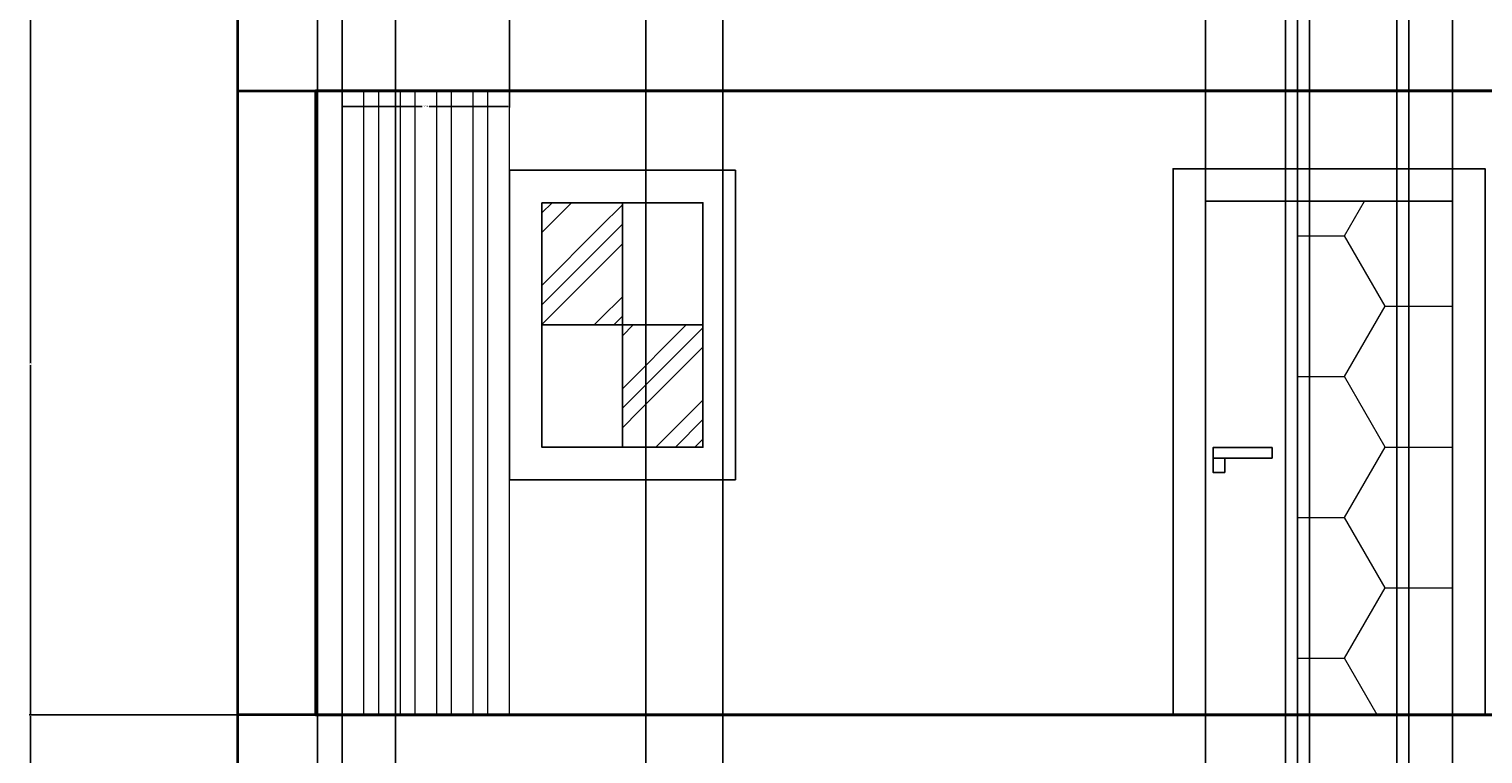
# Model space of a CAD drawing. Units: inches. Extents: x -8 to 554, y -200 to 499.
# Tile 6 of 12: x -8 to 216, y 121 to 233. Entities that reach past the tile are written whole.
import ezdxf

# ---------------------------------------------------------------- set-up
doc = ezdxf.new("R2010")
doc.units = ezdxf.units.IN
doc.header["$MEASUREMENT"] = 0
for name, color, linetype, lineweight in [('A-ANNO-DIMS', 2, 'Continuous', 18), ('A-DOOR', 3, 'Continuous', 25), ('A-DOOR-PATT', 252, 'Continuous', 13), ('A-FLOR', 7, 'Continuous', 35), ('A-GLAZ', 4, 'Continuous', 25), ('A-GLAZ-PATT', 252, 'Continuous', 13), ('A-WALL', 7, 'Continuous', 35), ('A-WALL-SCRN', 8, 'Continuous', 18)]:
    doc.layers.add(name, color=color, linetype=linetype, lineweight=lineweight)
doc.styles.get("Standard").update_dxf_attribs({"font": 'arial.ttf'})
doc.dimstyles.get("Standard").update_dxf_attribs({"dimtxt": 0.18, "dimasz": 0.18, "dimexe": 0.18, "dimexo": 0.0625, "dimgap": 0.09, "dimtad": 0, "dimtih": 1, "dimtoh": 1, "dimdec": 4, "dimzin": 0, "dimdsep": 46, "dimtxsty": 'Standard', "dimcen": 0.09, "dimadec": 0, "dimazin": 0, "dimtfac": 1, "dimtdec": 4, "dimtofl": 0, "dimtmove": 0, "dimatfit": 3, "dimfxl": 1, "dimtolj": 1, "dimtzin": 0, "dimarcsym": 0})

# ---------------------------------------------------------------- blocks, each defined once
blk = doc.blocks.new('DOOR-LEVER-ELEV')
for points in [[(0, 2.19), (9.08, 2.19), (9.08, 3.81), (0, 3.81)], [(0, 2.19), (1.8, 2.19), (1.8, 0), (0, 0)]]:
    blk.add_lwpolyline(points, close=True)
blk = doc.blocks.new('SCREEN-FIVE-FINS-ELEV')
for points in [[(0, 0), (3.37, 0), (3.37, 96), (0, 96)], [(5.59, 0), (8.97, 0), (8.97, 96), (5.59, 96)], [(11.19, 0), (14.56, 0), (14.56, 96), (11.19, 96)], [(16.78, 0), (20.16, 0), (20.16, 96), (16.78, 96)], [(22.38, 0), (25.75, 0), (25.75, 96), (22.38, 96)]]:
    blk.add_lwpolyline(points, close=True)
blk = doc.blocks.new('WINDOW-CASING-FOUR-LIGHT')
blk.add_lwpolyline([(0, 47.61), (34.77, 47.61), (34.77, 0), (0, 0)], close=True)
blk = doc.blocks.new('*D19')
at = {"layer": 'A-ANNO-DIMS', "color": 0, "lineweight": -2, "transparency": 16777216}
for p, q in [((40.45, 235.42), (40.45, 220.9)), ((66.2, 235.42), (66.2, 220.9)), ((40.63, 221.08), (52.8, 221.08)), ((66.02, 221.08), (53.86, 221.08))]:
    blk.add_line(p, q, dxfattribs=at)
at = {"layer": 'A-ANNO-DIMS', "color": 0, "transparency": 16777216}
for points in [[(40.63, 221.11), (40.63, 221.05), (40.45, 221.08)], [(66.02, 221.11), (66.02, 221.05), (66.2, 221.08)]]:
    blk.add_solid(points, dxfattribs=at)
at = {"layer": 'Defpoints', "color": 0, "transparency": 16777216}
for p in [(40.45, 235.48), (66.2, 235.48), (66.2, 221.08)]:
    blk.add_point(p, dxfattribs=at)
at = {"layer": 'A-ANNO-DIMS', "color": 0, "transparency": 16777216, "insert": (53.33, 221.08), "char_height": 0.18, "attachment_point": 5}
blk.add_mtext('\\A1;26 TYP.', dxfattribs=at)
blk = doc.blocks.new('*D31')
at = {"layer": 'A-ANNO-DIMS', "color": 0, "lineweight": -2, "transparency": 16777216}
for p, q in [((24.34, 127.42), (24.34, -199.97)), ((453.32, -30.73), (453.32, -199.97)), ((24.52, -199.79), (238.54, -199.79)), ((453.14, -199.79), (239.12, -199.79))]:
    blk.add_line(p, q, dxfattribs=at)
at = {"layer": 'A-ANNO-DIMS', "color": 0, "transparency": 16777216}
for points in [[(24.52, -199.76), (24.52, -199.82), (24.34, -199.79)], [(453.14, -199.76), (453.14, -199.82), (453.32, -199.79)]]:
    blk.add_solid(points, dxfattribs=at)
at = {"layer": 'Defpoints', "color": 0, "transparency": 16777216}
for p in [(24.34, 127.48), (453.32, -30.67), (453.32, -199.79)]:
    blk.add_point(p, dxfattribs=at)
at = {"layer": 'A-ANNO-DIMS', "color": 0, "transparency": 16777216, "insert": (238.83, -199.79), "char_height": 0.18, "attachment_point": 5}
blk.add_mtext('\\A1;429', dxfattribs=at)
blk = doc.blocks.new('*D32')
at = {"layer": 'A-ANNO-DIMS', "color": 0, "lineweight": -2, "transparency": 16777216}
for p, q in [((24.34, 223.42), (24.34, -199.97)), ((444.34, 223.42), (444.34, -199.97)), ((24.52, -199.79), (234.05, -199.79)), ((444.16, -199.79), (234.63, -199.79))]:
    blk.add_line(p, q, dxfattribs=at)
at = {"layer": 'A-ANNO-DIMS', "color": 0, "transparency": 16777216}
for points in [[(24.52, -199.76), (24.52, -199.82), (24.34, -199.79)], [(444.16, -199.76), (444.16, -199.82), (444.34, -199.79)]]:
    blk.add_solid(points, dxfattribs=at)
at = {"layer": 'Defpoints', "color": 0, "transparency": 16777216}
for p in [(24.34, 223.48), (444.34, 223.48), (444.34, -199.79)]:
    blk.add_point(p, dxfattribs=at)
at = {"layer": 'A-ANNO-DIMS', "color": 0, "transparency": 16777216, "insert": (234.34, -199.79), "char_height": 0.18, "attachment_point": 5}
blk.add_mtext('\\A1;420', dxfattribs=at)
blk = doc.blocks.new('*D34')
at = {"layer": 'A-ANNO-DIMS', "color": 0, "lineweight": -2, "transparency": 16777216}
for p, q in [((24.28, 127.48), (-7.69, 127.48)), ((-7.51, 127.3), (-7.51, 73.66)), ((-7.51, 19.66), (-7.51, 73.3)), ((36.28, 19.48), (-7.69, 19.48))]:
    blk.add_line(p, q, dxfattribs=at)
at = {"layer": 'A-ANNO-DIMS', "color": 0, "transparency": 16777216}
for points in [[(-7.54, 127.3), (-7.48, 127.3), (-7.51, 127.48)], [(-7.54, 19.66), (-7.48, 19.66), (-7.51, 19.48)]]:
    blk.add_solid(points, dxfattribs=at)
at = {"layer": 'Defpoints', "color": 0, "transparency": 16777216}
for p in [(-7.51, 127.48), (24.34, 127.48), (36.34, 19.48)]:
    blk.add_point(p, dxfattribs=at)
at = {"layer": 'A-ANNO-DIMS', "color": 0, "transparency": 16777216, "insert": (-7.51, 73.48), "char_height": 0.18, "attachment_point": 5}
blk.add_mtext('\\A1;108', dxfattribs=at)
blk = doc.blocks.new('*D35')
at = {"layer": 'A-ANNO-DIMS', "color": 0, "lineweight": -2, "transparency": 16777216}
for p, q in [((24.28, 235.48), (-7.69, 235.48)), ((-7.51, 235.3), (-7.51, 181.66)), ((-7.51, 127.66), (-7.51, 181.3)), ((24.28, 127.48), (-7.69, 127.48))]:
    blk.add_line(p, q, dxfattribs=at)
at = {"layer": 'A-ANNO-DIMS', "color": 0, "transparency": 16777216}
for points in [[(-7.54, 235.3), (-7.48, 235.3), (-7.51, 235.48)], [(-7.54, 127.66), (-7.48, 127.66), (-7.51, 127.48)]]:
    blk.add_solid(points, dxfattribs=at)
at = {"layer": 'Defpoints', "color": 0, "transparency": 16777216}
for p in [(-7.51, 235.48), (24.34, 235.48), (24.34, 127.48)]:
    blk.add_point(p, dxfattribs=at)
at = {"layer": 'A-ANNO-DIMS', "color": 0, "transparency": 16777216, "insert": (-7.51, 181.48), "char_height": 0.18, "attachment_point": 5}
blk.add_mtext('\\A1;108', dxfattribs=at)
blk = doc.blocks.new('*D41')
at = {"layer": 'A-ANNO-DIMS', "color": 0, "lineweight": -2, "transparency": 16777216}
for p, q in [((24.34, 235.42), (24.34, -199.97)), ((40.45, 235.42), (40.45, -199.97)), ((24.52, -199.79), (31.94, -199.79)), ((40.27, -199.79), (32.85, -199.79))]:
    blk.add_line(p, q, dxfattribs=at)
at = {"layer": 'A-ANNO-DIMS', "color": 0, "transparency": 16777216}
for points in [[(24.52, -199.76), (24.52, -199.82), (24.34, -199.79)], [(40.27, -199.76), (40.27, -199.82), (40.45, -199.79)]]:
    blk.add_solid(points, dxfattribs=at)
at = {"layer": 'Defpoints', "color": 0, "transparency": 16777216}
for p in [(24.34, 235.48), (40.45, 235.48), (40.45, -199.79)]:
    blk.add_point(p, dxfattribs=at)
at = {"layer": 'A-ANNO-DIMS', "color": 0, "transparency": 16777216, "insert": (32.4, -199.79), "char_height": 0.18, "attachment_point": 5}
blk.add_mtext('\\A1;16.113', dxfattribs=at)
blk = doc.blocks.new('*D55')
at = {"layer": 'A-ANNO-DIMS', "color": 0, "lineweight": -2, "transparency": 16777216}
for p, q in [((204.61, -30.61), (204.61, 498.99)), ((453.32, -30.61), (453.32, 498.99)), ((204.79, 498.81), (328.57, 498.81)), ((453.14, 498.81), (329.36, 498.81))]:
    blk.add_line(p, q, dxfattribs=at)
at = {"layer": 'A-ANNO-DIMS', "color": 0, "transparency": 16777216}
for points in [[(204.79, 498.84), (204.79, 498.78), (204.61, 498.81)], [(453.14, 498.84), (453.14, 498.78), (453.32, 498.81)]]:
    blk.add_solid(points, dxfattribs=at)
at = {"layer": 'Defpoints', "color": 0, "transparency": 16777216}
for p in [(453.32, 498.81), (204.61, -30.67), (453.32, -30.67)]:
    blk.add_point(p, dxfattribs=at)
at = {"layer": 'A-ANNO-DIMS', "color": 0, "transparency": 16777216, "insert": (328.96, 498.81), "char_height": 0.18, "attachment_point": 5}
blk.add_mtext('\\A1;248.7', dxfattribs=at)
blk = doc.blocks.new('*D56')
at = {"layer": 'A-ANNO-DIMS', "color": 0, "lineweight": -2, "transparency": 16777216}
for p, q in [((24.34, 7.54), (24.34, 498.99)), ((36.69, 7.54), (36.69, 498.99)), ((24.52, 498.81), (30.06, 498.81)), ((36.51, 498.81), (30.97, 498.81))]:
    blk.add_line(p, q, dxfattribs=at)
at = {"layer": 'A-ANNO-DIMS', "color": 0, "transparency": 16777216}
for points in [[(24.52, 498.84), (24.52, 498.78), (24.34, 498.81)], [(36.51, 498.84), (36.51, 498.78), (36.69, 498.81)]]:
    blk.add_solid(points, dxfattribs=at)
at = {"layer": 'Defpoints', "color": 0, "transparency": 16777216}
for p in [(36.69, 498.81), (24.34, 7.48), (36.69, 7.48)]:
    blk.add_point(p, dxfattribs=at)
at = {"layer": 'A-ANNO-DIMS', "color": 0, "transparency": 16777216, "insert": (30.52, 498.81), "char_height": 0.18, "attachment_point": 5}
blk.add_mtext('\\A1;12.346', dxfattribs=at)
blk = doc.blocks.new('*D57')
at = {"layer": 'A-ANNO-DIMS', "color": 0, "lineweight": -2, "transparency": 16777216}
for p, q in [((36.69, -52.46), (36.69, 498.99)), ((48.69, -52.46), (48.69, 498.99)), ((36.87, 498.81), (42.48, 498.81)), ((48.51, 498.81), (42.9, 498.81))]:
    blk.add_line(p, q, dxfattribs=at)
at = {"layer": 'A-ANNO-DIMS', "color": 0, "transparency": 16777216}
for points in [[(36.87, 498.84), (36.87, 498.78), (36.69, 498.81)], [(48.51, 498.84), (48.51, 498.78), (48.69, 498.81)]]:
    blk.add_solid(points, dxfattribs=at)
at = {"layer": 'Defpoints', "color": 0, "transparency": 16777216}
for p in [(48.69, 498.81), (36.69, -52.52), (48.69, -52.52)]:
    blk.add_point(p, dxfattribs=at)
at = {"layer": 'A-ANNO-DIMS', "color": 0, "transparency": 16777216, "insert": (42.69, 498.81), "char_height": 0.18, "attachment_point": 5}
blk.add_mtext('\\A1;12', dxfattribs=at)
blk = doc.blocks.new('*D58')
at = {"layer": 'A-ANNO-DIMS', "color": 0, "lineweight": -2, "transparency": 16777216}
for p, q in [((36.69, 7.54), (36.69, 498.99)), ((87.21, 7.54), (87.21, 498.99)), ((36.87, 498.81), (61.56, 498.81)), ((87.03, 498.81), (62.34, 498.81))]:
    blk.add_line(p, q, dxfattribs=at)
at = {"layer": 'A-ANNO-DIMS', "color": 0, "transparency": 16777216}
for points in [[(36.87, 498.84), (36.87, 498.78), (36.69, 498.81)], [(87.03, 498.84), (87.03, 498.78), (87.21, 498.81)]]:
    blk.add_solid(points, dxfattribs=at)
at = {"layer": 'Defpoints', "color": 0, "transparency": 16777216}
for p in [(87.21, 498.81), (36.69, 7.48), (87.21, 7.48)]:
    blk.add_point(p, dxfattribs=at)
at = {"layer": 'A-ANNO-DIMS', "color": 0, "transparency": 16777216, "insert": (61.95, 498.81), "char_height": 0.18, "attachment_point": 5}
blk.add_mtext('\\A1;50.52', dxfattribs=at)
blk = doc.blocks.new('*D59')
at = {"layer": 'A-ANNO-DIMS', "color": 0, "lineweight": -2, "transparency": 16777216}
for p, q in [((87.21, -60.84), (87.21, 498.99)), ((99.04, -60.84), (99.04, 498.99)), ((87.39, 498.81), (92.67, 498.81)), ((98.86, 498.81), (93.58, 498.81))]:
    blk.add_line(p, q, dxfattribs=at)
at = {"layer": 'A-ANNO-DIMS', "color": 0, "transparency": 16777216}
for points in [[(87.39, 498.84), (87.39, 498.78), (87.21, 498.81)], [(98.86, 498.84), (98.86, 498.78), (99.04, 498.81)]]:
    blk.add_solid(points, dxfattribs=at)
at = {"layer": 'Defpoints', "color": 0, "transparency": 16777216}
for p in [(99.04, 498.81), (87.21, -60.9), (99.04, -60.9)]:
    blk.add_point(p, dxfattribs=at)
at = {"layer": 'A-ANNO-DIMS', "color": 0, "transparency": 16777216, "insert": (93.12, 498.81), "char_height": 0.18, "attachment_point": 5}
blk.add_mtext('\\A1;11.827', dxfattribs=at)
blk = doc.blocks.new('*D60')
at = {"layer": 'A-ANNO-DIMS', "color": 0, "lineweight": -2, "transparency": 16777216}
for p, q in [((87.21, 7.54), (87.21, 498.99)), ((189.3, 7.54), (189.3, 498.99)), ((87.39, 498.81), (137.89, 498.81)), ((189.12, 498.81), (138.63, 498.81))]:
    blk.add_line(p, q, dxfattribs=at)
at = {"layer": 'A-ANNO-DIMS', "color": 0, "transparency": 16777216}
for points in [[(87.39, 498.84), (87.39, 498.78), (87.21, 498.81)], [(189.12, 498.84), (189.12, 498.78), (189.3, 498.81)]]:
    blk.add_solid(points, dxfattribs=at)
at = {"layer": 'Defpoints', "color": 0, "transparency": 16777216}
for p in [(189.3, 498.81), (87.21, 7.48), (189.3, 7.48)]:
    blk.add_point(p, dxfattribs=at)
at = {"layer": 'A-ANNO-DIMS', "color": 0, "transparency": 16777216, "insert": (138.26, 498.81), "char_height": 0.18, "attachment_point": 5}
blk.add_mtext('\\A1;102.1', dxfattribs=at)
blk = doc.blocks.new('*D61')
at = {"layer": 'A-ANNO-DIMS', "color": 0, "lineweight": -2, "transparency": 16777216}
for p, q in [((189.3, -52.46), (189.3, 498.99)), ((202.75, -52.46), (202.75, 498.99)), ((189.48, 498.81), (195.57, 498.81)), ((202.57, 498.81), (196.48, 498.81))]:
    blk.add_line(p, q, dxfattribs=at)
at = {"layer": 'A-ANNO-DIMS', "color": 0, "transparency": 16777216}
for points in [[(189.48, 498.84), (189.48, 498.78), (189.3, 498.81)], [(202.57, 498.84), (202.57, 498.78), (202.75, 498.81)]]:
    blk.add_solid(points, dxfattribs=at)
at = {"layer": 'Defpoints', "color": 0, "transparency": 16777216}
for p in [(202.75, 498.81), (189.3, -52.52), (202.75, -52.52)]:
    blk.add_point(p, dxfattribs=at)
at = {"layer": 'A-ANNO-DIMS', "color": 0, "transparency": 16777216, "insert": (196.03, 498.81), "char_height": 0.18, "attachment_point": 5}
blk.add_mtext('\\A1;13.446', dxfattribs=at)
blk = doc.blocks.new('*D62')
at = {"layer": 'A-ANNO-DIMS', "color": 0, "lineweight": -2, "transparency": 16777216}
for p, q in [((189.3, 7.54), (189.3, 498.99)), ((337.49, 7.54), (337.49, 498.99)), ((189.48, 498.81), (263.01, 498.81)), ((337.31, 498.81), (263.78, 498.81))]:
    blk.add_line(p, q, dxfattribs=at)
at = {"layer": 'A-ANNO-DIMS', "color": 0, "transparency": 16777216}
for points in [[(189.48, 498.84), (189.48, 498.78), (189.3, 498.81)], [(337.31, 498.84), (337.31, 498.78), (337.49, 498.81)]]:
    blk.add_solid(points, dxfattribs=at)
at = {"layer": 'Defpoints', "color": 0, "transparency": 16777216}
for p in [(337.49, 498.81), (189.3, 7.48), (337.49, 7.48)]:
    blk.add_point(p, dxfattribs=at)
at = {"layer": 'A-ANNO-DIMS', "color": 0, "transparency": 16777216, "insert": (263.4, 498.81), "char_height": 0.18, "attachment_point": 5}
blk.add_mtext('\\A1;148.2', dxfattribs=at)
blk = doc.blocks.new('*D80')
at = {"layer": 'A-ANNO-DIMS', "color": 0, "lineweight": -2, "transparency": 16777216}
for p, q in [((173.34, 314.42), (173.34, -199.97)), ((211.34, 314.42), (211.34, -199.97)), ((173.52, -199.79), (192.12, -199.79)), ((211.16, -199.79), (192.56, -199.79))]:
    blk.add_line(p, q, dxfattribs=at)
at = {"layer": 'A-ANNO-DIMS', "color": 0, "transparency": 16777216}
for points in [[(173.52, -199.76), (173.52, -199.82), (173.34, -199.79)], [(211.16, -199.76), (211.16, -199.82), (211.34, -199.79)]]:
    blk.add_solid(points, dxfattribs=at)
at = {"layer": 'Defpoints', "color": 0, "transparency": 16777216}
for p in [(173.34, 314.48), (211.34, 314.48), (211.34, -199.79)]:
    blk.add_point(p, dxfattribs=at)
at = {"layer": 'A-ANNO-DIMS', "color": 0, "transparency": 16777216, "insert": (192.34, -199.79), "char_height": 0.18, "attachment_point": 5}
blk.add_mtext('\\A1;38', dxfattribs=at)
blk = doc.blocks.new('*D81')
at = {"layer": 'A-ANNO-DIMS', "color": 0, "lineweight": -2, "transparency": 16777216}
for p, q in [((173.34, 235.42), (173.34, -199.97)), ((185.64, 235.42), (185.64, -199.97)), ((173.52, -199.79), (179.04, -199.79)), ((185.46, -199.79), (179.95, -199.79))]:
    blk.add_line(p, q, dxfattribs=at)
at = {"layer": 'A-ANNO-DIMS', "color": 0, "transparency": 16777216}
for points in [[(173.52, -199.76), (173.52, -199.82), (173.34, -199.79)], [(185.46, -199.76), (185.46, -199.82), (185.64, -199.79)]]:
    blk.add_solid(points, dxfattribs=at)
at = {"layer": 'Defpoints', "color": 0, "transparency": 16777216}
for p in [(173.34, 235.48), (185.64, 235.48), (185.64, -199.79)]:
    blk.add_point(p, dxfattribs=at)
at = {"layer": 'A-ANNO-DIMS', "color": 0, "transparency": 16777216, "insert": (179.49, -199.79), "char_height": 0.18, "attachment_point": 5}
blk.add_mtext('\\A1;12.302', dxfattribs=at)
blk = doc.blocks.new('*D82')
at = {"layer": 'A-ANNO-DIMS', "color": 0, "lineweight": -2, "transparency": 16777216}
for p, q in [((185.64, 235.42), (185.64, -199.97)), ((187.48, 235.42), (187.48, -199.97)), ((185.82, -199.79), (186.18, -199.79)), ((187.3, -199.79), (186.95, -199.79))]:
    blk.add_line(p, q, dxfattribs=at)
at = {"layer": 'A-ANNO-DIMS', "color": 0, "transparency": 16777216}
for points in [[(185.82, -199.76), (185.82, -199.82), (185.64, -199.79)], [(187.3, -199.76), (187.3, -199.82), (187.48, -199.79)]]:
    blk.add_solid(points, dxfattribs=at)
at = {"layer": 'Defpoints', "color": 0, "transparency": 16777216}
for p in [(185.64, 235.48), (187.48, 235.48), (187.48, -199.79)]:
    blk.add_point(p, dxfattribs=at)
at = {"layer": 'A-ANNO-DIMS', "color": 0, "transparency": 16777216, "insert": (186.56, -199.79), "char_height": 0.18, "attachment_point": 5}
blk.add_mtext('\\A1;1.837', dxfattribs=at)

msp = doc.modelspace()

# ---------------------------------------------------------------- hatches: boundary and pattern name
at = {"layer": 'A-DOOR-PATT', "transparency": 33554523}
h = msp.add_hatch(dxfattribs=at)
h.set_pattern_fill('HONEY', color=256, scale=100)
h.set_pattern_definition([(0, (-117.809, -80.312), (18.75, 10.82532), [12.5, -25]), (120, (-117.809, -80.312), (-18.75, 10.82532), [12.5, -25]), (60, (-117.809, -80.312), (4e-15, 21.65064), [-25, 12.5])])
h.paths.add_polyline_path([(211.3421, 314.4814), (187.4809, 314.4814), (187.4809, 235.4814), (211.3421, 235.4814)])
h.paths.add_polyline_path([(211.3421, 206.4814), (187.4809, 206.4814), (187.4809, 127.4814), (211.3421, 127.4814)])
h.paths.add_polyline_path([(211.3421, 98.4814), (187.4809, 98.4814), (187.4809, 19.4814), (211.3421, 19.4814)])
h.paths.add_polyline_path([(432.5174, 98.4814), (408.6562, 98.4814), (408.6562, 19.4814), (432.5174, 19.4814)])
h.paths.add_polyline_path([(432.5174, 206.4814), (408.6562, 206.4814), (408.6562, 127.4814), (432.5174, 127.4814), (432.5174, 155.7921)])
h.paths.add_polyline_path([(432.5174, 314.4814), (408.6562, 314.4814), (408.6562, 235.4814), (432.5174, 235.4814)])
at = {"layer": 'A-GLAZ-PATT'}
h = msp.add_hatch(dxfattribs=at)
h.set_pattern_fill('GOST_GROUND', color=256)
h.set_pattern_definition([(45, (-117.809, -80.312), (14.14214, 0), [20]), (45, (-114.809, -80.312), (14.14214, 0), [20]), (45, (-111.809, -80.312), (14.14214, 0), [20])])
h.paths.add_polyline_path([(83.5906, 206.2713), (71.2048, 206.2713), (71.2048, 187.4661), (83.5906, 187.4661)])
h.paths.add_polyline_path([(95.9765, 187.4661), (83.5906, 187.4661), (83.5906, 168.661), (95.9765, 168.661)])
h.paths.add_polyline_path([(83.5906, 98.2713), (71.2048, 98.2713), (71.2048, 79.4661), (83.5906, 79.4661)])
h.paths.add_polyline_path([(95.9765, 79.4661), (83.5906, 79.4661), (83.5906, 60.661), (95.9765, 60.661)])
h.paths.add_polyline_path([(333.2924, 98.788), (317.3421, 98.788), (317.3421, 61.7623), (333.2924, 61.7623)])
h.paths.add_polyline_path([(352.699, 98.788), (336.6386, 98.788), (336.6386, 61.7623), (352.699, 61.7623)])
h.paths.add_polyline_path([(333.2924, 206.788), (317.3421, 206.788), (317.3421, 169.7623), (333.2924, 169.7623)])
h.paths.add_polyline_path([(352.699, 206.788), (336.6386, 206.788), (336.6386, 169.7623), (352.699, 169.7623)])
h.paths.add_polyline_path([(333.2924, 314.788), (317.3421, 314.788), (317.3421, 277.7623), (333.2924, 277.7623)])
h.paths.add_polyline_path([(352.699, 314.788), (336.6386, 314.788), (336.6386, 277.7623), (352.699, 277.7623)])
h.paths.add_polyline_path([(95.9765, 295.4661), (83.5906, 295.4661), (83.5906, 276.661), (95.9765, 276.661)])
h.paths.add_polyline_path([(83.5906, 314.2713), (71.2048, 314.2713), (71.2048, 295.4661), (83.5906, 295.4661)])

# ---------------------------------------------------------------- linework, layer by layer
at = {"layer": 'A-DOOR'}
for p, q in [((173.3421, 127.4814), (173.3421, 206.4814)), ((173.3421, 206.4814), (211.3421, 206.4814)), ((211.3421, 206.4814), (211.3421, 127.4814))]:
    msp.add_line(p, q, dxfattribs=at)
for points in [[(216.3421, 127.4814), (168.3421, 127.4814), (168.3421, 211.4814), (216.3421, 211.4814)], [(185.644, 206.4814), (187.4809, 206.4814), (187.4809, 127.4814), (185.644, 127.4814)]]:
    msp.add_lwpolyline(points, close=True, dxfattribs=at)
at = {"layer": 'A-FLOR'}
for p, q in [((24.3421, 223.4814), (444.3421, 223.4814)), ((444.3421, 223.4814), (36.3421, 223.4814)), ((432.5174, 127.4814), (24.3421, 127.4814)), ((36.3421, 127.4814), (432.5174, 127.4814))]:
    msp.add_line(p, q, dxfattribs=at)
at = {"layer": 'A-GLAZ'}
for p, q in [((83.5906, 206.2713), (83.5906, 168.661)), ((71.2048, 187.4661), (95.9765, 187.4661))]:
    msp.add_line(p, q, dxfattribs=at)
msp.add_lwpolyline([(71.2048, 206.2713), (95.9765, 206.2713), (95.9765, 168.661), (71.2048, 168.661)], close=True, dxfattribs=at)
at = {"layer": 'A-WALL'}
for p, q in [((24.3421, 343.4814), (24.3421, 223.4814)), ((24.3421, 235.4814), (24.3421, 115.4814)), ((36.3421, 223.4814), (36.3421, 127.4814)), ((24.3421, 127.4814), (24.3421, 7.4814))]:
    msp.add_line(p, q, dxfattribs=at)

# ---------------------------------------------------------------- block references
at = {"layer": 'A-DOOR'}
msp.add_blockref('DOOR-LEVER-ELEV', (174.4762, 164.7884), dxfattribs=at)
at = {"layer": 'A-GLAZ'}
msp.add_blockref('WINDOW-CASING-FOUR-LIGHT', (66.2048, 163.661), dxfattribs=at)
at = {"layer": 'A-WALL-SCRN'}
msp.add_blockref('SCREEN-FIVE-FINS-ELEV', (40.4549, 127.4814), dxfattribs=at)

# ---------------------------------------------------------------- dimensions: what is measured, and where the dimension line sits
at = {"layer": 'A-ANNO-DIMS'}
for base, p1, p2, override, picture, middle in [((36.6882, 498.8091), (24.3421, 7.4814), (36.6882, 7.4814), {"dimdec": 3, "dimlfac": 1, "dimrnd": 0, "dimzin": 0, "dimdsep": 46, "dimlunit": 2}, '*D56', (30.5151, 498.8091)), ((48.6882, 498.8091), (36.6882, -52.5186), (48.6882, -52.5186), {"dimdec": 0, "dimlfac": 1, "dimrnd": 0, "dimzin": 0, "dimdsep": 46, "dimlunit": 2}, '*D57', (42.6882, 498.8091)), ((87.21, 498.8091), (36.6882, 7.4814), (87.21, 7.4814), {"dimdec": 2, "dimlfac": 1, "dimrnd": 0, "dimzin": 0, "dimdsep": 46, "dimlunit": 2}, '*D58', (61.9491, 498.8091)), ((99.037, 498.8091), (87.21, -60.9032), (99.037, -60.9032), {"dimdec": 3, "dimlfac": 1, "dimrnd": 0, "dimzin": 0, "dimdsep": 46, "dimlunit": 2}, '*D59', (93.1235, 498.8091)), ((189.3049, 498.8091), (87.21, 7.4814), (189.3049, 7.4814), {"dimdec": 1, "dimlfac": 1, "dimrnd": 0, "dimzin": 0, "dimdsep": 46, "dimlunit": 2}, '*D60', (138.2575, 498.8091)), ((202.7513, 498.8091), (189.3049, -52.5186), (202.7513, -52.5186), {"dimdec": 3, "dimlfac": 1, "dimrnd": 0, "dimzin": 0, "dimdsep": 46, "dimlunit": 2}, '*D61', (196.0281, 498.8091)), ((337.4923, 498.8091), (189.3049, 7.4814), (337.4923, 7.4814), {"dimdec": 1, "dimlfac": 1, "dimrnd": 0, "dimzin": 0, "dimdsep": 46, "dimlunit": 2}, '*D62', (263.3986, 498.8091)), ((453.3222, 498.8091), (204.6055, -30.6677), (453.3222, -30.6677), {"dimdec": 1, "dimlfac": 1, "dimrnd": 0, "dimzin": 0, "dimdsep": 46, "dimlunit": 2}, '*D55', (328.9639, 498.8091)), ((211.3421, -199.7912), (173.3421, 314.4814), (211.3421, 314.4814), {"dimdec": 0, "dimlfac": 1, "dimrnd": 0, "dimzin": 0, "dimdsep": 46, "dimlunit": 2}, '*D80', (192.3421, -199.7912)), ((40.4549, -199.7912), (24.3421, 235.4814), (40.4549, 235.4814), {"dimdec": 3, "dimlfac": 1, "dimrnd": 0, "dimzin": 0, "dimdsep": 46, "dimlunit": 2}, '*D41', (32.3985, -199.7912)), ((185.644, -199.7912), (173.3421, 235.4814), (185.644, 235.4814), {"dimdec": 3, "dimlfac": 1, "dimrnd": 0, "dimzin": 0, "dimdsep": 46, "dimlunit": 2}, '*D81', (179.493, -199.7912)), ((187.4809, -199.7912), (185.644, 235.4814), (187.4809, 235.4814), {"dimdec": 3, "dimlfac": 1, "dimrnd": 0, "dimzin": 0, "dimdsep": 46, "dimlunit": 2}, '*D82', (186.5625, -199.7912)), ((444.3421, -199.7912), (24.3421, 223.4814), (444.3421, 223.4814), {"dimdec": 0, "dimlfac": 1, "dimrnd": 0, "dimzin": 0, "dimdsep": 46, "dimlunit": 2}, '*D32', (234.3421, -199.7912)), ((453.3222, -199.7912), (24.3421, 127.4814), (453.3222, -30.6677), {"dimdec": 0, "dimlfac": 1, "dimrnd": 0, "dimzin": 0, "dimdsep": 46, "dimlunit": 2}, '*D31', (238.8321, -199.7912))]:
    dim = msp.add_linear_dim(base=base, p1=p1, p2=p2, dimstyle='Standard', override=override, dxfattribs=at)
    dim.commit()
    dim.dimension.update_dxf_attribs({"geometry": picture, "text_midpoint": middle})
for base, p1, p2, picture, middle in [((-7.5079, 235.4814), (24.3421, 127.4814), (24.3421, 235.4814), '*D35', (-7.5079, 181.4814)), ((-7.5079, 127.4814), (36.3421, 19.4814), (24.3421, 127.4814), '*D34', (-7.5079, 73.4814))]:
    dim = msp.add_linear_dim(base=base, p1=p1, p2=p2, angle=90, dimstyle='Standard', override={"dimdec": 0, "dimlfac": 1, "dimrnd": 0, "dimzin": 0, "dimdsep": 46, "dimlunit": 2}, dxfattribs=at)
    dim.commit()
    dim.dimension.update_dxf_attribs({"geometry": picture, "text_midpoint": middle})
dim = msp.add_linear_dim(base=(66.2048, 221.0814), p1=(40.4549, 235.4814), p2=(66.2048, 235.4814), text='<> TYP.', dimstyle='Standard', override={"dimdec": 0, "dimlfac": 1, "dimrnd": 0, "dimzin": 0, "dimdsep": 46, "dimlunit": 2}, dxfattribs=at)
dim.commit()
dim.dimension.update_dxf_attribs({"geometry": '*D19', "text_midpoint": (53.3298, 221.0814)})

doc.saveas('drawing.dxf')
